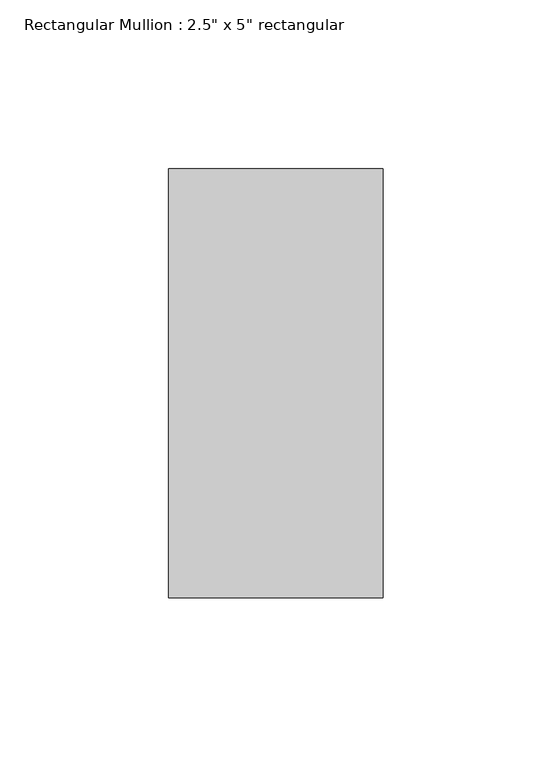
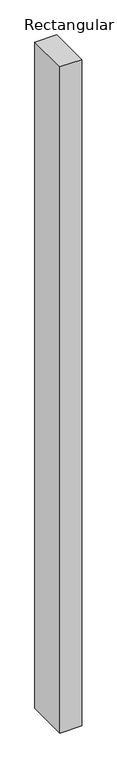
"""IFC4 building model written with IfcOpenShell, lengths in millimetres: member geometry."""

from ifc_helpers import new_model, si_unit, frame, origin, place, context, project, spatial, polyline, outline, extrude, source, transform, mapped, element, save


def member_8ea2817a(model_context):
    return source(origin(), model_context, "Body", "SweptSolid", [
        extrude(outline(polyline([(31.75, 63.5), (31.75, -63.5), (-31.75, -63.5), (-31.75, 63.5), (31.75, 63.5)])), frame((0.0, 0.0, -2063.6147749), z_axis=(0.0, 0.0, 1.0), x_axis=(1.0, 0.0, 0.0)), (0.0, 0.0, 1.0), 2063.6147749),
    ])


if __name__ == "__main__":
    model = new_model("IFC4")
    model_context = context("Model", 3, world=origin())
    ifc_project = project(units=[si_unit("LENGTHUNIT", "METRE", prefix="MILLI")], contexts=[model_context])
    site = spatial("IfcSite", under=ifc_project)
    building = spatial("IfcBuilding", under=site)
    placement = place(None, origin())
    member_shape = member_8ea2817a(model_context)
    element("IfcMember", 1, ObjectType="Rectangular Mullion : 2.5\" x 5\" rectangular", at=placement, inside=building, context=model_context, shape_type="MappedRepresentation", body=[
        mapped(member_shape, transform((0.0, 0.0, 0.0), x_axis=(1.0, 0.0, 0.0), y_axis=(0.0, 1.0, 0.0), z_axis=(0.0, 0.0, 1.0))),
    ])
    save(model, "model.ifc")

# Revit data of these elements
# Type "Rectangular Mullion : 2.5\" x 5\" rectangular"
#   built-in parameter 1007304 = 0.416667 (stored number, unit not read)
#   built-in parameter 1007301 = 0.104167 (stored number, unit not read)
#   built-in parameter 1007300 = 0.104167 (stored number, unit not read)
# Element 1 (IfcMember, "Rectangular Mullion : 2.5\" x 5\" rectangular")
#   Materials on its faces: "Aluminum"
# Materials
#   "Aluminum": class "Metal", colour RGB 247 247 247, transparency 0, Description = "Aluminum 6061", Cost = 0
